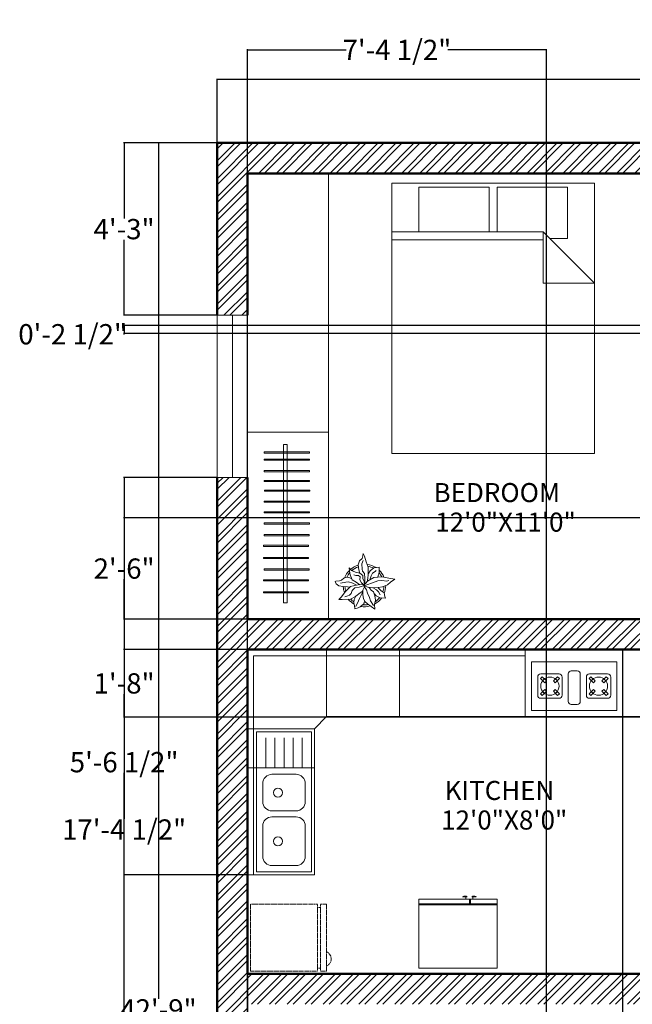
# Model space of a CAD drawing. Units: inches. Extents: x -71 to 434, y -519 to 67.
# Tile 4 of 7: x -71 to 110, y -224 to 67. Entities that reach past the tile are written whole.
import ezdxf

# ---------------------------------------------------------------- set-up
doc = ezdxf.new("R2010")
doc.units = ezdxf.units.IN
doc.header["$MEASUREMENT"] = 0
doc.linetypes.add('HIDDEN', pattern=[0.375, 0.25, -0.125])
for name, color, linetype, lineweight in [('A-ANNO-DIMS', 7, 'Continuous', 18), ('A-AREA-IDEN', 7, 'Continuous', 25), ('A-EQPM', 21, 'Continuous', 18), ('A-EQPM-HIDN', 21, 'HIDDEN', 18), ('A-FLOR-CASE', 9, 'Continuous', 18), ('A-FLOR-FIXT', 9, 'Continuous', 18), ('A-WALL-PATT', 8, 'Continuous', 13), ('CAY', 94, 'Continuous', 13), ('FURNITURE', 5, 'Continuous', 18), ('WALL', 50, 'Continuous', 50), ('WINDOW', 1, 'Continuous', 18)]:
    doc.layers.add(name, color=color, linetype=linetype, lineweight=lineweight)
doc.styles.add('ATT', font='romans.shx')
doc.styles.get("Standard").update_dxf_attribs({"font": 'arial.ttf'})
doc.dimstyles.get("Standard").update_dxf_attribs({"dimtxt": 6, "dimasz": 0.18, "dimexe": 0.18, "dimexo": 0.0625, "dimgap": 0.09, "dimtad": 0, "dimtih": 1, "dimtoh": 1, "dimdec": 0, "dimzin": 0, "dimdsep": 46, "dimlunit": 3, "dimtxsty": 'Standard', "dimcen": 0.09, "dimadec": 0, "dimazin": 0, "dimtfac": 1, "dimtdec": 0, "dimtofl": 0, "dimtmove": 0, "dimatfit": 3, "dimfxl": 1, "dimtolj": 1, "dimtzin": 0, "dimarcsym": 0})

# ---------------------------------------------------------------- blocks, each defined once
blk = doc.blocks.new('Bed - Queen')
for p, q in [((0, -80.00003), (0, 0)), ((0, 0), (59.99999, 0)), ((59.99999, 0), (59.99999, -80.00003)), ((7.99999, -1.2), (28.79998, -1.2)), ((7.99999, -14.4), (7.99999, -1.2)), ((28.79998, -1.2), (28.79998, -14.4)), ((31.19999, -1.2), (51.99999, -1.2)), ((31.19999, -14.4), (31.19999, -1.2)), ((51.99999, -1.2), (51.99999, -16.4)), ((0, -14.4), (44.8, -14.4)), ((59.99999, -29.6), (44.8, -14.4)), ((44.8, -14.4), (44.8, -29.6)), ((44.8, -16.8), (0, -16.8)), ((51.99999, -16.4), (46.79936, -16.4)), ((44.8, -29.6), (59.99999, -29.6)), ((59.99999, -80.00003), (0, -80.00003))]:
    blk.add_line(p, q)
blk = doc.blocks.new('*D17')
at = {"layer": 'A-ANNO-DIMS', "color": 0, "lineweight": -2, "transparency": 16777216}
for p, q in [((-12.59, 30.9), (-12.59, 49.86)), ((-12.41, 49.68), (180.23, 49.68)), ((383.23, 49.68), (190.59, 49.68)), ((383.41, 30.9), (383.41, 49.86))]:
    blk.add_line(p, q, dxfattribs=at)
at = {"layer": 'A-ANNO-DIMS', "color": 0, "transparency": 16777216}
for points in [[(-12.41, 49.71), (-12.41, 49.65), (-12.59, 49.68)], [(383.23, 49.71), (383.23, 49.65), (383.41, 49.68)]]:
    blk.add_solid(points, dxfattribs=at)
at = {"layer": 'Defpoints', "color": 0, "transparency": 16777216}
for p in [(383.41, 49.68), (-12.59, 30.83), (383.41, 30.83)]:
    blk.add_point(p, dxfattribs=at)
at = {"layer": 'A-ANNO-DIMS', "color": 0, "transparency": 16777216, "insert": (185.41, 49.68), "char_height": 6, "attachment_point": 5}
blk.add_mtext("\\A1;33'", dxfattribs=at)
blk = doc.blocks.new('*D18')
at = {"layer": 'A-ANNO-DIMS', "color": 0, "lineweight": -2, "transparency": 16777216}
for p, q in [((-12.65, 30.83), (-30.15, 30.83)), ((-29.97, 30.65), (-29.97, -222.51)), ((-29.97, -481.99), (-29.97, -228.82)), ((-12.65, -482.17), (-30.15, -482.17))]:
    blk.add_line(p, q, dxfattribs=at)
at = {"layer": 'A-ANNO-DIMS', "color": 0, "transparency": 16777216}
for points in [[(-30, 30.65), (-29.94, 30.65), (-29.97, 30.83)], [(-30, -481.99), (-29.94, -481.99), (-29.97, -482.17)]]:
    blk.add_solid(points, dxfattribs=at)
at = {"layer": 'Defpoints', "color": 0, "transparency": 16777216}
for p in [(-12.59, 30.83), (-29.97, -482.17), (-12.59, -482.17)]:
    blk.add_point(p, dxfattribs=at)
at = {"layer": 'A-ANNO-DIMS', "color": 0, "transparency": 16777216, "insert": (-29.97, -225.67), "char_height": 6, "attachment_point": 5}
blk.add_mtext('\\A1;42\'-9"', dxfattribs=at)
blk = doc.blocks.new('12PPLT12')
at = {"color": 0, "linetype": 'ByBlock'}
for p, q in [((-0.034, 0.694), (-0.032, 0.751)), ((-0.032, 0.751), (-0.002, 0.689)), ((-0.148, 0.486), (-0.116, 0.583)), ((-0.132, 0.367), (-0.148, 0.486)), ((-0.116, 0.583), (-0.05, 0.632)), ((-0.064, 0.51), (-0.026, 0.591)), ((-0.05, 0.38), (-0.064, 0.51)), ((-0.05, 0.632), (-0.034, 0.694)), ((-0.002, 0.689), (0.044, 0.559)), ((0.044, 0.559), (0.09, 0.432)), ((-0.349, 0.334), (-0.362, 0.415)), ((-0.362, 0.415), (-0.303, 0.35)), ((-0.332, 0.247), (-0.349, 0.334)), ((-0.289, 0.136), (-0.332, 0.247)), ((-0.303, 0.35), (-0.208, 0.312)), ((-0.205, 0.231), (-0.251, 0.247)), ((-0.208, 0.312), (-0.105, 0.29)), ((-0.108, 0.279), (-0.132, 0.367)), ((-0.105, 0.29), (-0.037, 0.236)), ((-0.043, 0.334), (-0.05, 0.38)), ((0.003, 0.279), (-0.043, 0.334)), ((-0.037, 0.236), (-0.034, 0.158)), ((0.009, 0.169), (0.003, 0.279)), ((0.09, 0.253), (0.082, 0.174)), ((0.09, 0.432), (0.09, 0.339)), ((0.09, 0.339), (0.09, 0.253)), ((0.093, 0.282), (0.134, 0.347)), ((0.134, 0.347), (0.22, 0.415)), ((0.193, 0.293), (0.155, 0.228)), ((0.25, 0.328), (0.193, 0.293)), ((0.22, 0.415), (0.291, 0.421)), ((0.28, 0.353), (0.25, 0.328)), ((0.291, 0.421), (0.35, 0.429)), ((0.342, 0.266), (0.304, 0.19)), ((0.348, 0.331), (0.342, 0.266)), ((0.35, 0.429), (0.348, 0.331)), ((-0.671, 0.098), (-0.687, 0.095)), ((-0.687, 0.095), (-0.666, 0.036)), ((-0.59, 0.109), (-0.671, 0.098)), ((-0.666, 0.036), (-0.601, -0.005)), ((-0.536, 0.125), (-0.59, 0.109)), ((-0.563, 0.052), (-0.441, 0.074)), ((-0.487, 0.171), (-0.536, 0.125)), ((-0.425, 0.193), (-0.487, 0.171)), ((-0.441, 0.074), (-0.373, 0.084)), ((-0.346, 0.179), (-0.425, 0.193)), ((-0.373, 0.084), (-0.27, 0.057)), ((-0.292, 0.149), (-0.346, 0.179)), ((-0.229, 0.003), (-0.324, -0.027)), ((-0.194, 0.074), (-0.289, 0.136)), ((-0.27, 0.057), (-0.186, 0.006)), ((-0.069, 0.027), (-0.229, 0.003)), ((-0.137, 0.231), (-0.205, 0.231)), ((-0.108, 0.019), (-0.194, 0.074)), ((-0.097, 0.204), (-0.137, 0.231)), ((-0.01, 0.003), (-0.121, -0.038)), ((-0.11, 0.133), (-0.097, 0.204)), ((-0.069, 0.06), (-0.11, 0.133)), ((-0.01, 0.014), (-0.069, 0.06)), ((-0.002, 0.006), (-0.069, 0.027)), ((-0.034, 0.158), (-0.007, 0.101)), ((-0.018, -0.008), (0.074, 0.098)), ((-0.01, -0.005), (0.169, 0.055)), ((0.003, 0.017), (-0.01, 0.014)), ((0.003, -0.029), (-0.01, 0.003)), ((-0.007, 0.101), (0.003, 0.017)), ((0.006, 0.027), (0.009, 0.169)), ((0.082, 0.174), (0.061, 0.082)), ((0.074, 0.098), (0.223, 0.188)), ((0.155, 0.228), (0.131, 0.13)), ((0.169, 0.055), (0.315, 0.109)), ((0.223, 0.188), (0.421, 0.204)), ((0.315, 0.109), (0.413, 0.117)), ((0.413, 0.117), (0.524, 0.101)), ((0.421, 0.204), (0.573, 0.171)), ((0.545, 0.017), (0.429, -0.032)), ((0.524, 0.101), (0.578, 0.114)), ((0.613, 0.074), (0.545, 0.017)), ((0.573, 0.171), (0.716, 0.152)), ((0.716, 0.152), (0.613, 0.074)), ((-0.601, -0.005), (-0.503, -0.021)), ((-0.452, -0.152), (-0.536, -0.268)), ((-0.503, -0.021), (-0.4, -0.032)), ((-0.395, -0.094), (-0.452, -0.152)), ((-0.4, -0.032), (-0.357, -0.04)), ((-0.324, -0.027), (-0.395, -0.094)), ((-0.352, -0.227), (-0.387, -0.241)), ((-0.316, -0.187), (-0.352, -0.227)), ((-0.292, -0.122), (-0.316, -0.187)), ((-0.224, -0.059), (-0.292, -0.122)), ((-0.121, -0.038), (-0.224, -0.059)), ((-0.213, -0.263), (-0.135, -0.195)), ((-0.135, -0.195), (-0.053, -0.14)), ((-0.119, -0.304), (-0.04, -0.148)), ((-0.053, -0.14), (0.003, -0.029)), ((-0.037, -0.122), (-0.04, -0.219)), ((-0.04, -0.219), (-0.021, -0.308)), ((0.082, -0.038), (-0.018, -0.008)), ((-0.007, -0.024), (0.05, -0.105)), ((0.05, -0.105), (0.071, -0.181)), ((0.071, -0.181), (0.12, -0.282)), ((0.188, -0.054), (0.082, -0.038)), ((0.112, -0.051), (0.09, -0.043)), ((0.155, -0.108), (0.112, -0.051)), ((0.212, -0.152), (0.155, -0.108)), ((0.323, -0.051), (0.188, -0.054)), ((0.247, -0.246), (0.212, -0.152)), ((0.215, -0.062), (0.282, -0.103)), ((0.234, -0.2), (0.277, -0.241)), ((0.282, -0.103), (0.334, -0.146)), ((0.429, -0.032), (0.323, -0.051)), ((0.396, -0.124), (0.326, -0.054)), ((0.334, -0.146), (0.372, -0.217)), ((0.464, -0.176), (0.396, -0.124)), ((0.48, -0.257), (0.464, -0.176)), ((-0.536, -0.268), (-0.606, -0.328)), ((-0.606, -0.328), (-0.522, -0.328)), ((-0.522, -0.328), (-0.324, -0.325)), ((-0.387, -0.241), (-0.465, -0.268)), ((-0.324, -0.325), (-0.213, -0.263)), ((-0.244, -0.33), (-0.247, -0.406)), ((-0.247, -0.406), (-0.233, -0.471)), ((-0.193, -0.236), (-0.244, -0.33)), ((-0.199, -0.494), (-0.139, -0.358)), ((-0.139, -0.358), (-0.119, -0.304)), ((-0.102, -0.503), (-0.017, -0.432)), ((-0.021, -0.308), (0.006, -0.376)), ((-0.017, -0.432), (0.003, -0.378)), ((0.006, -0.376), (0.074, -0.428)), ((0.074, -0.428), (0.158, -0.496)), ((0.12, -0.282), (0.139, -0.363)), ((0.139, -0.363), (0.212, -0.474)), ((0.236, -0.444), (0.261, -0.349)), ((0.242, -0.561), (0.236, -0.444)), ((0.261, -0.349), (0.247, -0.246)), ((0.277, -0.241), (0.372, -0.287)), ((0.372, -0.287), (0.494, -0.301)), ((0.494, -0.301), (0.48, -0.257)), ((-0.233, -0.471), (-0.222, -0.551)), ((-0.222, -0.551), (-0.148, -0.522)), ((-0.148, -0.522), (-0.102, -0.503)), ((0.158, -0.496), (0.242, -0.561))]:
    blk.add_line(p, q, dxfattribs=at)
for radius, start, end in [(0.5, 107.123, 130.9816), (0.5, 56.9563, 82.295), (0.5, 134.8021, 159.1804), (0.458, 138.4756, 155.3347), (0.458, 107.9864, 130.5771), (0.458, 62.6899, 79.5345), (0.458, 26.2761, 41.1349), (0.5, 22.9768, 45.8473), (0.5, 182.503, 200.4563), (0.458, 183.2699, 197.4002), (0.458, 340.6559, 357.5057), (0.5, 338.5862, 359.7442), (0.5, 220.6606, 241.3393), (0.458, 225.0835, 237.5023), (0.458, 264.1886, 282.4028), (0.5, 298.3455, 324.4541), (0.458, 303.3868, 322.0756), (0.5, 259.7038, 286.1281)]:
    blk.add_arc((0, 0), radius, start, end, dxfattribs=at)
at = {"color": 0, "linetype": 'ByBlock', "style": 'ATT'}
for tag, p, flags in [('ITEM', (-1, -3.25), 3), ('ROOM_NUMBER', (-1, -4.583), 1)]:
    blk.add_attdef(tag, p, '', height=1, dxfattribs=dict(at, flags=flags))
blk = doc.blocks.new('WIN-48x9')
blk.add_line((0, 4.5), (48, 4.5))
blk.add_lwpolyline([(0, 0), (48, 0), (48, 9), (0, 9)], close=True)
blk = doc.blocks.new('WARDROBE-HANGING-BAY')
blk.add_line((24, 50.57), (0, 50.57))
for points in [[(10.65, 46.88), (11.71, 46.88), (11.71, 0), (10.65, 0)], [(4.96, 44.68), (18.35, 44.68), (18.35, 44.35), (4.96, 44.35)], [(4.96, 42.56), (18.35, 42.56), (18.35, 42.22), (4.96, 42.22)], [(18.35, 38.84), (4.96, 38.84), (4.96, 39.17), (18.35, 39.17)], [(4.96, 36.28), (18.35, 36.28), (18.35, 35.95), (4.96, 35.95)], [(18.43, 33.04), (5.05, 33.04), (5.05, 33.37), (18.43, 33.37)], [(4.96, 30.15), (18.35, 30.15), (18.35, 29.82), (4.96, 29.82)], [(18.33, 26.66), (4.95, 26.66), (4.95, 26.99), (18.33, 26.99)], [(4.96, 23.69), (18.35, 23.69), (18.35, 23.36), (4.96, 23.36)], [(18.29, 19.89), (4.91, 19.89), (4.91, 20.22), (18.29, 20.22)], [(4.71, 17.05), (18.09, 17.05), (18.09, 16.72), (4.71, 16.72)], [(18.09, 13.11), (4.71, 13.11), (4.71, 13.44), (18.09, 13.44)], [(18.29, 9.72), (4.91, 9.72), (4.91, 10.05), (18.29, 10.05)], [(4.71, 6.88), (18.09, 6.88), (18.09, 6.55), (4.71, 6.55)], [(18.09, 2.94), (4.71, 2.94), (4.71, 3.27), (18.09, 3.27)]]:
    blk.add_lwpolyline(points, close=True)
blk = doc.blocks.new('*D44')
at = {"layer": 'A-ANNO-DIMS', "color": 0, "lineweight": -2, "transparency": 16777216}
for p, q in [((-12.65, 30.83), (-40.32, 30.83)), ((-40.14, 30.65), (-40.14, 8.49)), ((-40.14, -19.99), (-40.14, 2.18)), ((-12.65, -20.17), (-40.32, -20.17))]:
    blk.add_line(p, q, dxfattribs=at)
at = {"layer": 'A-ANNO-DIMS', "color": 0, "transparency": 16777216}
for points in [[(-40.17, 30.65), (-40.11, 30.65), (-40.14, 30.83)], [(-40.17, -19.99), (-40.11, -19.99), (-40.14, -20.17)]]:
    blk.add_solid(points, dxfattribs=at)
at = {"layer": 'Defpoints', "color": 0, "transparency": 16777216}
for p in [(-12.59, 30.83), (-40.14, -20.17), (-12.59, -20.17)]:
    blk.add_point(p, dxfattribs=at)
at = {"layer": 'A-ANNO-DIMS', "color": 0, "transparency": 16777216, "insert": (-40.14, 5.33), "char_height": 6, "attachment_point": 5}
blk.add_mtext('\\A1;4\'-3"', dxfattribs=at)
blk = doc.blocks.new('*D45')
at = {"layer": 'A-ANNO-DIMS', "color": 0, "lineweight": -2, "transparency": 16777216}
for p, q in [((-12.65, -68.17), (-40.32, -68.17)), ((-40.14, -68.35), (-40.14, -169.22)), ((-40.14, -276.49), (-40.14, -175.61)), ((-12.65, -276.67), (-40.32, -276.67))]:
    blk.add_line(p, q, dxfattribs=at)
at = {"layer": 'A-ANNO-DIMS', "color": 0, "transparency": 16777216}
for points in [[(-40.17, -68.35), (-40.11, -68.35), (-40.14, -68.17)], [(-40.17, -276.49), (-40.11, -276.49), (-40.14, -276.67)]]:
    blk.add_solid(points, dxfattribs=at)
at = {"layer": 'Defpoints', "color": 0, "transparency": 16777216}
for p in [(-12.59, -68.17), (-40.14, -276.67), (-12.59, -276.67)]:
    blk.add_point(p, dxfattribs=at)
at = {"layer": 'A-ANNO-DIMS', "color": 0, "transparency": 16777216, "insert": (-40.14, -172.42), "char_height": 6, "attachment_point": 5}
blk.add_mtext('\\A1;17\'-4 1/2"', dxfattribs=at)
blk = doc.blocks.new('*D46')
at = {"layer": 'A-ANNO-DIMS', "color": 0, "lineweight": -2, "transparency": 16777216}
for p, q in [((-3.59, -368.1), (-3.59, 58.56)), ((-3.41, 58.38), (25.63, 58.38)), ((84.73, 58.38), (55.69, 58.38)), ((84.91, -368.1), (84.91, 58.56))]:
    blk.add_line(p, q, dxfattribs=at)
at = {"layer": 'A-ANNO-DIMS', "color": 0, "transparency": 16777216}
for points in [[(-3.41, 58.41), (-3.41, 58.35), (-3.59, 58.38)], [(84.73, 58.41), (84.73, 58.35), (84.91, 58.38)]]:
    blk.add_solid(points, dxfattribs=at)
at = {"layer": 'Defpoints', "color": 0, "transparency": 16777216}
for p in [(84.91, 58.38), (-3.59, -368.17), (84.91, -368.17)]:
    blk.add_point(p, dxfattribs=at)
at = {"layer": 'A-ANNO-DIMS', "color": 0, "transparency": 16777216, "insert": (40.66, 58.38), "char_height": 6, "attachment_point": 5}
blk.add_mtext('\\A1;7\'-4 1/2"', dxfattribs=at)
blk = doc.blocks.new('*D59')
at = {"layer": 'A-ANNO-DIMS', "color": 0, "lineweight": -2, "transparency": 16777216}
for p, q in [((149.35, -80.17), (-40.32, -80.17)), ((-40.14, -80.35), (-40.14, -92.01)), ((-40.14, -109.99), (-40.14, -98.32)), ((149.35, -110.17), (-40.32, -110.17))]:
    blk.add_line(p, q, dxfattribs=at)
at = {"layer": 'A-ANNO-DIMS', "color": 0, "transparency": 16777216}
for points in [[(-40.17, -80.35), (-40.11, -80.35), (-40.14, -80.17)], [(-40.17, -109.99), (-40.11, -109.99), (-40.14, -110.17)]]:
    blk.add_solid(points, dxfattribs=at)
at = {"layer": 'Defpoints', "color": 0, "transparency": 16777216}
for p in [(149.41, -80.17), (-40.14, -110.17), (149.41, -110.17)]:
    blk.add_point(p, dxfattribs=at)
at = {"layer": 'A-ANNO-DIMS', "color": 0, "transparency": 16777216, "insert": (-40.14, -95.17), "char_height": 6, "attachment_point": 5}
blk.add_mtext('\\A1;2\'-6"', dxfattribs=at)
blk = doc.blocks.new('*D60')
at = {"layer": 'A-ANNO-DIMS', "color": 0, "lineweight": -2, "transparency": 16777216}
for p, q in [((149.35, -23.17), (-40.32, -23.17)), ((149.35, -25.61), (-40.32, -25.61)), ((-40.14, -25.79), (-40.32, -25.79)), ((-40.14, -23.35), (-40.14, -25.43)), ((-40.14, -25.61), (-40.14, -25.79))]:
    blk.add_line(p, q, dxfattribs=at)
at = {"layer": 'A-ANNO-DIMS', "color": 0, "transparency": 16777216}
for points in [[(-40.17, -23.35), (-40.11, -23.35), (-40.14, -23.17)], [(-40.17, -25.43), (-40.11, -25.43), (-40.14, -25.61)]]:
    blk.add_solid(points, dxfattribs=at)
at = {"layer": 'Defpoints', "color": 0, "transparency": 16777216}
for p in [(149.41, -23.17), (-40.14, -25.61), (149.41, -25.61)]:
    blk.add_point(p, dxfattribs=at)
at = {"layer": 'A-ANNO-DIMS', "color": 0, "transparency": 16777216, "insert": (-55.38, -25.79), "char_height": 6, "attachment_point": 5}
blk.add_mtext('\\A1;0\'-2 1/2"', dxfattribs=at)
blk = doc.blocks.new('*D64')
at = {"layer": 'A-ANNO-DIMS', "color": 0, "lineweight": -2, "transparency": 16777216}
for p, q in [((320.35, -119.17), (-40.32, -119.17)), ((-40.14, -119.35), (-40.14, -126)), ((-40.14, -138.97), (-40.14, -132.31)), ((320.35, -139.15), (-40.32, -139.15))]:
    blk.add_line(p, q, dxfattribs=at)
at = {"layer": 'A-ANNO-DIMS', "color": 0, "transparency": 16777216}
for points in [[(-40.17, -119.35), (-40.11, -119.35), (-40.14, -119.17)], [(-40.17, -138.97), (-40.11, -138.97), (-40.14, -139.15)]]:
    blk.add_solid(points, dxfattribs=at)
at = {"layer": 'Defpoints', "color": 0, "transparency": 16777216}
for p in [(320.41, -119.17), (-40.14, -139.15), (320.41, -139.15)]:
    blk.add_point(p, dxfattribs=at)
at = {"layer": 'A-ANNO-DIMS', "color": 0, "transparency": 16777216, "insert": (-40.14, -129.16), "char_height": 6, "attachment_point": 5}
blk.add_mtext('\\A1;1\'-8"', dxfattribs=at)
blk = doc.blocks.new('*D66')
at = {"layer": 'A-ANNO-DIMS', "color": 0, "lineweight": -2, "transparency": 16777216}
for p, q in [((-3.59, -119.23), (-3.59, -509.9)), ((107.49, -119.23), (107.49, -509.9)), ((-3.41, -509.72), (43.89, -509.72)), ((107.31, -509.72), (60.02, -509.72))]:
    blk.add_line(p, q, dxfattribs=at)
at = {"layer": 'A-ANNO-DIMS', "color": 0, "transparency": 16777216}
for points in [[(-3.41, -509.69), (-3.41, -509.75), (-3.59, -509.72)], [(107.31, -509.69), (107.31, -509.75), (107.49, -509.72)]]:
    blk.add_solid(points, dxfattribs=at)
at = {"layer": 'Defpoints', "color": 0, "transparency": 16777216}
for p in [(-3.59, -119.17), (107.49, -119.17), (107.49, -509.72)]:
    blk.add_point(p, dxfattribs=at)
at = {"layer": 'A-ANNO-DIMS', "color": 0, "transparency": 16777216, "insert": (51.95, -509.72), "char_height": 6, "attachment_point": 5}
blk.add_mtext('\\A1;9\'-3"', dxfattribs=at)
blk = doc.blocks.new('*D67')
at = {"layer": 'A-ANNO-DIMS', "color": 0, "lineweight": -2, "transparency": 16777216}
for p, q in [((107.56, -119.17), (411.14, -119.17)), ((410.96, -119.35), (410.96, -125.92)), ((410.96, -138.8), (410.96, -132.22)), ((107.56, -138.98), (411.14, -138.98))]:
    blk.add_line(p, q, dxfattribs=at)
at = {"layer": 'A-ANNO-DIMS', "color": 0, "transparency": 16777216}
for points in [[(410.93, -119.35), (410.99, -119.35), (410.96, -119.17)], [(410.93, -138.8), (410.99, -138.8), (410.96, -138.98)]]:
    blk.add_solid(points, dxfattribs=at)
at = {"layer": 'Defpoints', "color": 0, "transparency": 16777216}
for p in [(107.49, -119.17), (107.49, -138.98), (410.96, -138.98)]:
    blk.add_point(p, dxfattribs=at)
at = {"layer": 'A-ANNO-DIMS', "color": 0, "transparency": 16777216, "insert": (410.96, -129.07), "char_height": 6, "attachment_point": 5}
blk.add_mtext('\\A1;1\'-8"', dxfattribs=at)
blk = doc.blocks.new('*D68')
at = {"layer": 'A-ANNO-DIMS', "color": 0, "lineweight": -2, "transparency": 16777216}
for p, q in [((-3.65, -119.17), (-40.32, -119.17)), ((-40.14, -119.35), (-40.14, -149.29)), ((-40.14, -185.62), (-40.14, -155.67)), ((-3.65, -185.8), (-40.32, -185.8))]:
    blk.add_line(p, q, dxfattribs=at)
at = {"layer": 'A-ANNO-DIMS', "color": 0, "transparency": 16777216}
for points in [[(-40.17, -119.35), (-40.11, -119.35), (-40.14, -119.17)], [(-40.17, -185.62), (-40.11, -185.62), (-40.14, -185.8)]]:
    blk.add_solid(points, dxfattribs=at)
at = {"layer": 'Defpoints', "color": 0, "transparency": 16777216}
for p in [(-3.59, -119.17), (-40.14, -185.8), (-3.59, -185.8)]:
    blk.add_point(p, dxfattribs=at)
at = {"layer": 'A-ANNO-DIMS', "color": 0, "transparency": 16777216, "insert": (-40.14, -152.48), "char_height": 6, "attachment_point": 5}
blk.add_mtext('\\A1;5\'-6 1/2"', dxfattribs=at)
blk = doc.blocks.new('*D75')
at = {"layer": 'A-ANNO-DIMS', "color": 0, "lineweight": -2, "transparency": 16777216}
for p, q in [((225.52, -80.17), (-40.32, -80.17)), ((-40.14, -80.35), (-40.14, -92.01)), ((-40.14, -109.99), (-40.14, -98.32)), ((221.35, -110.17), (-40.32, -110.17))]:
    blk.add_line(p, q, dxfattribs=at)
at = {"layer": 'A-ANNO-DIMS', "color": 0, "transparency": 16777216}
for points in [[(-40.17, -80.35), (-40.11, -80.35), (-40.14, -80.17)], [(-40.17, -109.99), (-40.11, -109.99), (-40.14, -110.17)]]:
    blk.add_solid(points, dxfattribs=at)
at = {"layer": 'Defpoints', "color": 0, "transparency": 16777216}
for p in [(225.58, -80.17), (-40.14, -110.17), (221.41, -110.17)]:
    blk.add_point(p, dxfattribs=at)
at = {"layer": 'A-ANNO-DIMS', "color": 0, "transparency": 16777216, "insert": (-40.14, -95.17), "char_height": 6, "attachment_point": 5}
blk.add_mtext('\\A1;2\'-6"', dxfattribs=at)

msp = doc.modelspace()

# ---------------------------------------------------------------- hatches: boundary and pattern name
at = {"layer": 'A-WALL-PATT'}
h = msp.add_hatch(dxfattribs=at)
h.set_pattern_fill('ANSI32', color=256, scale=10)
h.set_pattern_definition([(45, (-213.138, 0), (-2.65165, 2.65165), []), (45, (-211.37, 0), (-2.65165, 2.65165), [])])
h.paths.add_polyline_path([(383.41, 30.83), (230.41, 30.83), (149.41, 30.83), (-12.59, 30.83), (-12.59, -20.17), (-3.59, -20.17), (-3.59, 21.83), (140.41, 21.83), (140.41, 15.83), (149.41, 15.83), (149.41, 21.83), (221.41, 21.83), (221.41, 15.83), (230.41, 15.83), (230.41, 21.83), (374.41, 21.83), (374.41, -110.17), (369.41, -110.17), (369.41, -119.17), (374.41, -119.17), (374.41, -215.17), (320.41, -215.17), (320.41, -119.17), (345.41, -119.17), (345.41, -110.17), (221.41, -110.17), (221.41, -119.17), (311.41, -119.17), (311.41, -215.17), (192.42, -215.17), (192.42, -224.17), (221.41, -224.17), (221.41, -228.23), (230.41, -228.23), (230.41, -224.17), (374.41, -224.17), (374.41, -368.17), (230.41, -368.17), (230.41, -266.34), (221.41, -266.34), (221.41, -368.17), (192.08, -368.17), (192.08, -377.17), (230.41, -377.17), (374.41, -377.17), (374.41, -473.17), (230.41, -473.17), (212.41, -473.17), (212.41, -482.17), (383.41, -482.17), (383.41, -377.17), (383.41, -224.17), (383.41, -119.17)])
h.paths.add_polyline_path([(149.41, -110.17), (-3.59, -110.17), (-3.59, -68.17), (-12.59, -68.17), (-12.59, -276.67), (-3.59, -276.67), (-3.59, -224.17), (154.41, -224.17), (154.41, -215.17), (149.41, -215.17), (149.41, -154.17), (140.41, -154.17), (140.41, -215.17), (-3.59, -215.17), (-3.59, -119.17), (19.82, -119.17), (140.41, -119.17), (140.41, -124.17), (149.41, -124.17)])
h.paths.add_polyline_path([(84.91, -368.17), (-3.59, -368.17), (-3.59, -324.67), (-12.59, -324.67), (-12.59, -377.17), (-12.59, -401.17), (-3.59, -401.17), (-3.59, -377.17), (84.91, -377.17)], flags=17)
h.paths.add_polyline_path([(1.41, -473.17), (-3.59, -473.17), (-3.59, -468.17), (-12.59, -468.17), (-12.59, -482.17), (1.41, -482.17)], flags=17)

# ---------------------------------------------------------------- linework, layer by layer
at = {"layer": 'A-EQPM'}
for points in [[(80.56, -137.17), (80.56, -122.77), (105.77, -122.77), (105.77, -137.17)], [(84.94, -128.44), (83.67, -127.17), (83.16, -127.68), (84.43, -128.95)], [(86.98, -128.44), (88.25, -127.17), (88.76, -127.68), (87.49, -128.95)], [(99.35, -128.44), (98.08, -127.17), (97.57, -127.68), (98.84, -128.95)], [(101.39, -128.44), (102.66, -127.17), (103.17, -127.68), (101.9, -128.95)], [(84.94, -131.5), (83.67, -132.77), (83.16, -132.26), (84.43, -130.99)], [(86.98, -131.5), (88.25, -132.77), (88.76, -132.26), (87.49, -130.99)], [(99.35, -131.5), (98.08, -132.77), (97.57, -132.26), (98.84, -130.99)], [(101.39, -131.5), (102.66, -132.77), (103.17, -132.26), (101.9, -130.99)]]:
    msp.add_lwpolyline(points, close=True, dxfattribs=at)
for points in [[(88.66, -133.57), (83.26, -133.57, -0.414214), (82.36, -132.67), (82.36, -127.27, -0.414214), (83.26, -126.37), (88.66, -126.37, -0.414214), (89.56, -127.27), (89.56, -132.67, -0.414214)], [(94.07, -135.37), (92.27, -135.37, -0.414214), (91.37, -134.47), (91.37, -126.37, -0.414214), (92.27, -125.47), (94.07, -125.47, -0.414214), (94.97, -126.37), (94.97, -134.47, -0.414214)], [(97.67, -133.57), (103.07, -133.57, 0.414214), (103.97, -132.67), (103.97, -127.27, 0.414214), (103.07, -126.37), (97.67, -126.37, 0.414214), (96.77, -127.27), (96.77, -132.67, 0.414214)]]:
    msp.add_lwpolyline(points, format="xyb", close=True, dxfattribs=at)
for centre in [(85.96, -129.97), (100.37, -129.97)]:
    msp.add_circle(centre, 2.7, dxfattribs=at)
for points, invisible_edges in [([(62.13, -193.02, 2.72), (47.15, -193.02, 2.72), (62.13, -193.02, 44.95)], 2), ([(47.15, -193.02, 44.95), (62.13, -193.02, 44.95), (47.15, -193.02, 2.72)], 2), ([(47.15, -194.38, 44.95), (47.15, -193.02, 44.95), (47.15, -194.38, 2.72)], 2), ([(47.15, -193.02, 2.72), (47.15, -194.38, 2.72), (47.15, -193.02, 44.95)], 2), ([(47.15, -194.38, 44.95), (62.13, -194.38, 44.95), (47.15, -193.02, 44.95)], 2), ([(62.13, -193.02, 44.95), (47.15, -193.02, 44.95), (62.13, -194.38, 44.95)], 2), ([(47.15, -213.45), (47.15, -213.45, 44.95), (47.15, -194.72)], 2), ([(47.15, -194.72, 44.95), (47.15, -194.72), (47.15, -213.45, 44.95)], 2), ([(70.3, -194.72), (47.15, -194.72), (70.3, -194.72, 2.72)], 2), ([(47.15, -194.72, 2.72), (70.3, -194.72, 2.72), (47.15, -194.72)], 2), ([(47.15, -213.45, 44.95), (70.3, -213.45, 44.95), (47.15, -194.72, 44.95)], 2), ([(70.3, -194.72, 44.95), (47.15, -194.72, 44.95), (70.3, -213.45, 44.95)], 2), ([(70.3, -193.02, 2.72), (62.47, -193.02, 2.72), (70.3, -193.02, 44.95)], 2), ([(62.47, -193.02, 44.95), (70.3, -193.02, 44.95), (62.47, -193.02, 2.72)], 2), ([(70.3, -194.38, 44.95), (70.3, -193.02, 44.95), (62.47, -194.38, 44.95)], 2), ([(62.47, -193.02, 44.95), (62.47, -194.38, 44.95), (70.3, -193.02, 44.95)], 2), ([(70.3, -193.02, 44.95), (70.3, -194.38, 44.95), (70.3, -194.38, 2.72)], 12), ([(70.3, -194.38, 2.72), (70.3, -193.02, 2.72), (70.3, -193.02, 44.95)], 12), ([(70.3, -213.45, 44.95), (70.3, -213.45), (70.3, -194.72)], 12), ([(70.3, -194.72), (70.3, -194.72, 44.95), (70.3, -213.45, 44.95)], 12), ([(47.15, -213.45), (70.3, -213.45), (47.15, -213.45, 44.95)], 2), ([(70.3, -213.45, 44.95), (47.15, -213.45, 44.95), (70.3, -213.45)], 2)]:
    msp.add_3dface(points, dxfattribs=dict(at, invisible_edges=invisible_edges))
at = {"layer": 'A-EQPM-HIDN'}
for p, q in [((18.02, -214.37), (18.02, -194.56)), ((18.02, -194.56), (19.82, -194.56)), ((19.82, -194.56), (19.82, -214.37)), ((18.02, -195.46), (17.12, -195.46)), ((18.02, -213.47), (17.12, -213.47)), ((19.82, -214.37), (18.02, -214.37))]:
    msp.add_line(p, q, dxfattribs=at)
msp.add_lwpolyline([(-2.69, -214.37), (17.12, -214.37), (17.12, -194.56), (-2.69, -194.56)], close=True, dxfattribs=at)
msp.add_arc((18.81, -210.74), 2.37, 295.0923, 64.9077, dxfattribs=at)
at = {"layer": 'A-FLOR-CASE'}
for p, q in [((20.41, 21.83), (20.41, -110.17)), ((19.82, -120.97), (41.43, -120.97)), ((41.43, -120.97), (78.68, -120.97)), ((41.43, -138.98), (78.68, -138.98)), ((-1.79, -185.8), (-1.79, -142.58))]:
    msp.add_line(p, q, dxfattribs=at)
for points in [[(16.22, -142.58), (-3.59, -142.58), (-3.59, -119.17), (19.82, -119.17), (19.82, -138.98)], [(19.82, -138.98), (19.82, -119.17), (41.43, -119.17), (41.43, -138.98)], [(78.68, -138.98), (78.68, -119.17), (107.49, -119.17), (107.49, -138.98)], [(16.22, -185.8), (-3.59, -185.8), (-3.59, -142.58), (16.22, -142.58)]]:
    msp.add_lwpolyline(points, close=True, dxfattribs=at)
msp.add_lwpolyline([(-1.79, -142.58), (-1.79, -120.97), (19.82, -120.97)], dxfattribs=at)
at = {"layer": 'A-FLOR-FIXT'}
for p, q in [((1.81, -154.28), (1.81, -145.28)), ((4.51, -154.28), (4.51, -145.28)), ((4.51, -154.28), (4.51, -145.28)), ((7.21, -154.28), (7.21, -145.28)), ((9.91, -154.28), (9.91, -145.28)), ((12.62, -154.28), (12.62, -145.28)), ((-3.59, -154.17), (16.22, -154.17))]:
    msp.add_line(p, q, dxfattribs=at)
msp.add_lwpolyline([(15.32, -184.9), (-0.89, -184.9), (-0.89, -143.48), (15.32, -143.48)], close=True, dxfattribs=at)
for points in [[(0.91, -164.19, 0.414214), (3.61, -166.89), (10.82, -166.89, 0.414214), (13.52, -164.19), (13.52, -158.79, 0.414214), (10.82, -156.08), (3.61, -156.08, 0.414214), (0.91, -158.79)], [(0.91, -180.4, 0.414214), (3.61, -183.1), (10.82, -183.1, 0.414214), (13.52, -180.4), (13.52, -171.39, 0.414214), (10.82, -168.69), (3.61, -168.69, 0.414214), (0.91, -171.39)]]:
    msp.add_lwpolyline(points, format="xyb", close=True, dxfattribs=at)
for centre in [(5.41, -161.49), (5.41, -175.89)]:
    msp.add_circle(centre, 1.35, dxfattribs=at)
at = {"layer": 'WALL'}
for p, q in [((-12.59, 30.83), (149.41, 30.83)), ((-12.59, 30.83), (-12.59, -20.17)), ((-3.59, 21.83), (140.41, 21.83)), ((-3.59, 21.83), (-3.59, -20.17)), ((-12.59, -68.17), (-12.59, -276.67)), ((-3.59, -68.17), (-3.59, -110.17)), ((-3.59, -110.17), (149.41, -110.17)), ((-3.59, -119.17), (140.41, -119.17)), ((-3.59, -119.17), (-3.59, -215.17)), ((-3.59, -215.17), (140.41, -215.17))]:
    msp.add_line(p, q, dxfattribs=at)

# ---------------------------------------------------------------- block references
at = {"layer": 'A-FLOR-CASE'}
msp.add_blockref('WARDROBE-HANGING-BAY', (-3.59, -105.33), dxfattribs=at)
at = {"layer": 'CAY', "xscale": 12.58515090877727, "yscale": 12.58515090877727, "zscale": 12.58515090877727}
msp.add_blockref('12PPLT12', (31.03, -100.17), dxfattribs=at)
at = {"layer": 'FURNITURE'}
msp.add_blockref('Bed - Queen', (39.19, 18.91), dxfattribs=at)
at = {"layer": 'WINDOW', "rotation": 90.00000000000007}
msp.add_blockref('WIN-48x9', (-3.59, -68.17), dxfattribs=at)

# ---------------------------------------------------------------- texts
at = {"layer": 'A-AREA-IDEN'}
for s, height, p in [('BEDROOM', 5.643, (51.51, -75.49)), ('12\'0"X11\'0"', 5.6432, (52.01, -84.24)), ('KITCHEN', 5.643, (54.8, -163.67)), ('12\'0"X8\'0"', 5.643, (53.76, -172.43))]:
    msp.add_text(s, height=height, dxfattribs=at).set_placement(p)

# ---------------------------------------------------------------- dimensions: what is measured, and where the dimension line sits
at = {"layer": 'A-ANNO-DIMS'}
for base, p1, p2, override, picture, middle in [((84.91, 58.38), (-3.59, -368.17), (84.91, -368.17), {"dimdec": 1, "dimlfac": 1, "dimrnd": 0, "dimzin": 1, "dimdsep": 46, "dimlunit": 4, "dimfrac": 2}, '*D46', (40.66, 58.38)), ((383.41, 49.68), (-12.59, 30.83), (383.41, 30.83), {"dimclrd": 0, "dimclre": 0, "dimclrt": 0}, '*D17', (185.41, 49.68)), ((107.49, -509.72), (-3.59, -119.17), (107.49, -119.17), {"dimdec": 1, "dimlfac": 1, "dimrnd": 0, "dimzin": 1, "dimdsep": 46, "dimlunit": 4, "dimfrac": 2}, '*D66', (51.95, -509.72))]:
    dim = msp.add_linear_dim(base=base, p1=p1, p2=p2, dimstyle='Standard', override=override, dxfattribs=at)
    dim.commit()
    dim.dimension.update_dxf_attribs({"geometry": picture, "text_midpoint": middle})
for base, p1, p2, override, picture, middle in [((-40.14, -20.17), (-12.59, 30.83), (-12.59, -20.17), {"dimdec": 1, "dimlfac": 1, "dimrnd": 0, "dimzin": 1, "dimdsep": 46, "dimlunit": 4, "dimfrac": 2}, '*D44', (-40.14, 5.33)), ((-29.97, -482.17), (-12.59, 30.83), (-12.59, -482.17), {"dimclrd": 0, "dimclre": 0, "dimclrt": 0}, '*D18', (-29.97, -225.67)), ((-40.14, -25.61), (149.41, -23.17), (149.41, -25.61), {"dimdec": 1, "dimlfac": 1, "dimrnd": 0, "dimzin": 1, "dimdsep": 46, "dimlunit": 4, "dimfrac": 2}, '*D60', (-55.38, -25.79)), ((-40.14, -276.67), (-12.59, -68.17), (-12.59, -276.67), {"dimdec": 1, "dimlfac": 1, "dimrnd": 0, "dimzin": 1, "dimdsep": 46, "dimlunit": 4, "dimfrac": 2}, '*D45', (-40.14, -172.42)), ((-40.14, -110.17), (149.41, -80.17), (149.41, -110.17), {"dimdec": 1, "dimlfac": 1, "dimrnd": 0, "dimzin": 1, "dimdsep": 46, "dimlunit": 4, "dimfrac": 2}, '*D59', (-40.14, -95.17)), ((-40.14, -110.17), (225.58, -80.17), (221.41, -110.17), {"dimdec": 1, "dimlfac": 1, "dimrnd": 0, "dimzin": 1, "dimdsep": 46, "dimlunit": 4, "dimfrac": 2}, '*D75', (-40.14, -95.17)), ((-40.14, -185.8), (-3.59, -119.17), (-3.59, -185.8), {"dimdec": 1, "dimlfac": 1, "dimrnd": 0, "dimzin": 1, "dimdsep": 46, "dimlunit": 4, "dimfrac": 2}, '*D68', (-40.14, -152.48)), ((-40.14, -139.15), (320.41, -119.17), (320.41, -139.15), {"dimdec": 1, "dimlfac": 1, "dimrnd": 0, "dimzin": 1, "dimdsep": 46, "dimlunit": 4, "dimfrac": 2}, '*D64', (-40.14, -129.16)), ((410.96, -138.98), (107.49, -119.17), (107.49, -138.98), {"dimdec": 1, "dimlfac": 1, "dimrnd": 0, "dimzin": 1, "dimdsep": 46, "dimlunit": 4, "dimfrac": 2}, '*D67', (410.96, -129.07))]:
    dim = msp.add_linear_dim(base=base, p1=p1, p2=p2, angle=90, dimstyle='Standard', override=override, dxfattribs=at)
    dim.commit()
    dim.dimension.update_dxf_attribs({"geometry": picture, "text_midpoint": middle})

# ---------------------------------------------------------------- meshes
at = {"layer": 'A-EQPM'}
mesh = msp.add_polyface(dxfattribs=at)
corners = [(61.45, -192.34, 21.79), (60.09, -192.34, 21.79), (60.09, -192.34, 34.05), (61.45, -192.34, 34.05), (61.12, -192.18, 21.79), (61.12, -192.18, 34.05), (60.83, -192.18, 21.79), (60.83, -192.18, 34.05), (60.49, -192.18, 21.79), (60.49, -192.18, 34.05), (60.23, -192.21, 21.79), (60.23, -192.21, 34.05), (64.17, -192.34, 21.79), (62.81, -192.34, 21.79), (64.17, -192.34, 34.05), (62.81, -192.34, 34.05), (63.13, -192.18, 21.79), (63.13, -192.18, 34.05), (63.43, -192.18, 21.79), (63.43, -192.18, 34.05), (63.76, -192.18, 21.79), (63.76, -192.18, 34.05), (64.03, -192.21, 21.79), (64.03, -192.21, 34.05), (63.15, -193.02, 34.05), (63.15, -192.34, 34.05), (63.15, -193.02, 21.79), (63.15, -192.34, 21.79), (61.11, -193.02, 34.05), (61.11, -192.34, 34.05), (61.11, -193.02, 21.79), (61.11, -192.34, 21.79)]
mesh.append_faces([[corners[k] for k in face] for face in [(3, 0, 2), (5, 4, 3), (7, 6, 5), (9, 8, 7), (11, 10, 9), (2, 1, 11), (12, 13, 14), (15, 13, 14), (13, 16, 15), (16, 18, 17), (18, 20, 19), (20, 22, 21), (22, 12, 23), (24, 25, 26), (27, 26, 25), (28, 29, 30), (31, 30, 29), (15, 14, 13), (12, 13, 14)]], dxfattribs={"vtx1": -1})
mesh.append_faces([[corners[k] for k in face] for face in [(0, 1, 2), (4, 0, 3), (6, 4, 5), (8, 6, 7), (10, 8, 9), (1, 10, 11), (16, 17, 15), (18, 19, 17), (20, 21, 19), (22, 23, 21), (12, 14, 23), (3, 2, 1), (1, 0, 3)]], dxfattribs={"vtx2": -1})
mesh = msp.add_polyface(dxfattribs=at)
corners = [(62.13, -193.02, 44.95), (62.47, -193.02, 44.95), (62.47, -193.02, 2.72), (62.13, -193.02, 2.72), (62.13, -194.38, 44.95), (62.47, -194.38, 44.95), (47.15, -194.72, 44.95), (47.15, -194.38, 44.95), (47.15, -194.38, 2.72), (47.15, -194.72, 2.72), (70.3, -194.72, 44.95), (70.3, -194.38, 44.95), (70.3, -194.72, 2.72), (70.3, -194.38, 2.72)]
mesh.append_faces([[corners[k] for k in face] for face in [(4, 5, 0), (1, 0, 5), (10, 11, 6), (7, 6, 11)]], dxfattribs={"vtx1": -1})
mesh.append_faces([[corners[k] for k in face] for face in [(0, 1, 2), (2, 3, 0), (6, 7, 8), (8, 9, 6), (12, 13, 11), (11, 10, 12)]], dxfattribs={"vtx2": -1})

doc.saveas('drawing.dxf')
